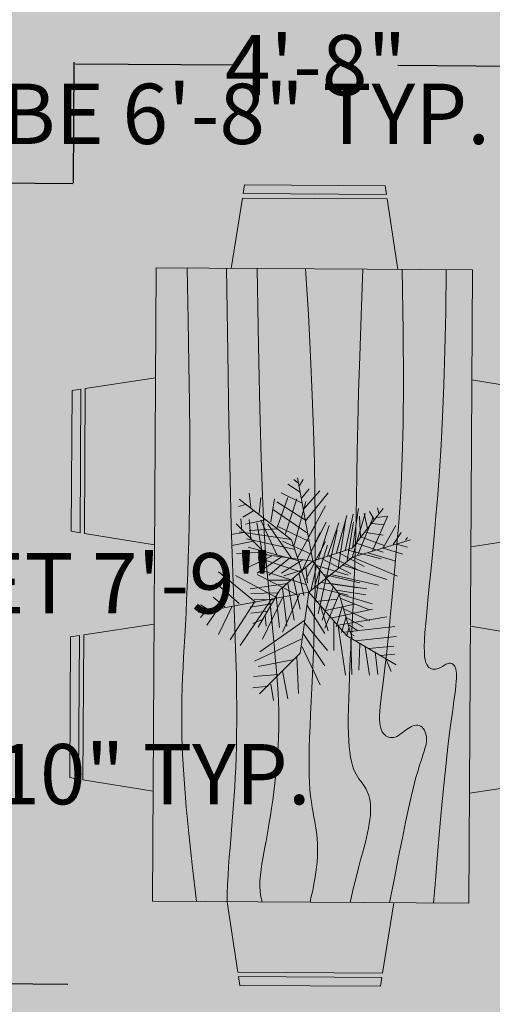
# Model space of a CAD drawing. Units: inches. Extents: x 1316 to 1777, y 813 to 1650.
# Tile 9 of 22: x 1512 to 1567, y 1319 to 1434. Entities that reach past the tile are written whole.
import ezdxf

# ---------------------------------------------------------------- set-up
doc = ezdxf.new("R2010")
doc.units = ezdxf.units.IN
doc.header["$MEASUREMENT"] = 0
for name, color, linetype, lineweight in [('A-ANNO-DIMS', 2, 'Continuous', 18), ('A-FURN-PATT', 23, 'Continuous', 13), ('furniture', 23, 'Continuous', 18), ('greenary', 106, 'Continuous', 13)]:
    doc.layers.add(name, color=color, linetype=linetype, lineweight=lineweight)
doc.layers.add('A-FLOR-PATT', color=254, linetype='Continuous', lineweight=13, true_color=0xfeeab9)
doc.styles.get("Standard").update_dxf_attribs({"font": 'arial.ttf'})
doc.dimstyles.get("Standard").update_dxf_attribs({"dimtxt": 7, "dimasz": 0.18, "dimexe": 0.18, "dimexo": 0.0625, "dimgap": 0.09, "dimtad": 0, "dimtih": 1, "dimtoh": 1, "dimzin": 0, "dimdsep": 46, "dimlunit": 3, "dimtxsty": 'Standard', "dimcen": 0.09, "dimadec": 0, "dimazin": 0, "dimtfac": 1, "dimtofl": 0, "dimtmove": 0, "dimatfit": 3, "dimfxl": 1, "dimtolj": 1, "dimtzin": 0, "dimarcsym": 0})

# ---------------------------------------------------------------- blocks, each defined once
blk = doc.blocks.new('*U13')
for p, q in [((-10.186, 53.64), (-13.084, 55.962)), ((0, 0), (-10.5, 57)), ((-9.099, 51.782), (-6.563, 55.962)), ((-8.737, 47.138), (-17.069, 52.711)), ((-7.288, 39.707), (-21.778, 46.673)), ((-7.65, 43.423), (-2.578, 49.46)), ((-5.839, 35.992), (4.667, 48.067)), ((-5.114, 27.632), (10.463, 46.673)), ((-5.114, 28.097), (-24.676, 40.636)), ((-2.941, 16.486), (8.652, 37.85)), ((27, 9), (48, 36)), ((27.127, 9.056), (31.112, 35.992)), ((44.153, 36.456), (45.239, 32.741)), ((-3.665, 19.273), (-27.574, 35.527)), ((16.259, 5.805), (23.142, 31.348)), ((22.055, 7.198), (27.489, 32.277)), ((31.836, 30.883), (32.561, 16.486)), ((35.096, 32.741), (37.27, 22.524)), ((38.719, 34.134), (41.979, 28.561)), ((43.791, 29.954), (51.036, 30.883)), ((-31.5, 4.5), (-52.5, 25.5)), ((-48.585, 21.131), (-49.309, 29.026)), ((-43.513, 28.561), (-42.427, 15.558)), ((-38.442, 26.239), (-34.819, 7.663)), ((-35.544, 28.097), (-24.314, 3.947)), ((-1.129, 6.734), (9.014, 26.704)), ((10.101, 3.483), (17.708, 26.239)), ((40.53, 25.775), (48.862, 24.846)), ((-14.533, 2.09), (-30.834, 25.31)), ((-24.314, 23.917), (-2.941, 13.7)), ((3.942, 1.625), (11.187, 24.381)), ((-47.498, 19.737), (-55.83, 18.344)), ((33.285, 16.486), (48.862, 10.913)), ((36.183, 19.737), (48.137, 17.88)), ((-40.615, 13.7), (-55.105, 10.913)), ((-20.691, 13.7), (-1.129, 4.876)), ((29.662, 12.307), (48.137, 6.269)), ((-33.37, 6.269), (-52.207, 5.34)), ((0, 0), (27, 9)), ((18.07, 5.805), (35.096, -3.483)), ((24.229, 7.663), (46.688, 1.625)), ((-28.299, 3.483), (-47.86, -5.805)), ((-21.416, 3.018), (-38.079, -8.128)), ((0, 0), (-31.5, 4.5)), ((-15.982, 2.09), (-30.11, -9.521)), ((0, 0), (-22.5, -19.5)), ((-6.563, 1.161), (-21.416, -8.128)), ((0, 0), (18, -22.5)), ((6.478, 1.625), (26.04, -8.592)), ((11.187, 3.483), (30.749, -5.805)), ((-4.752, -3.483), (-3.665, -14.629)), ((2.493, -3.019), (-1.491, -20.202)), ((1.769, -2.555), (24.229, -9.521)), ((-6.563, -5.805), (-19.967, -9.985)), ((-9.461, -8.592), (-6.201, -23.453)), ((5.029, -6.27), (2.131, -25.775)), ((7.565, -9.056), (32.198, -14.629)), ((-17.431, -15.094), (-42.789, -18.809)), ((-15.257, -12.772), (-30.11, -12.772)), ((-17.069, -15.094), (-12.721, -40.172)), ((-13.446, -11.378), (-8.737, -32.741)), ((9.014, -11.378), (3.58, -35.992)), ((12.274, -15.094), (36.907, -18.809)), ((-22.5, -19.5), (-37.5, -45)), ((-20.691, -18.345), (-17.793, -44.352)), ((14.085, -16.951), (6.478, -40.172)), ((16.259, -19.738), (36.183, -22.989)), ((-24.314, -21.596), (-42.427, -22.06)), ((-25.038, -23.918), (-22.865, -45.281)), ((18.07, -22.524), (8.289, -45.745)), ((18, -22.5), (27, -52.5)), ((18.433, -22.524), (40.53, -29.026)), ((19.157, -25.311), (38.719, -33.206)), ((-28.299, -29.026), (-42.789, -31.348)), ((-26.849, -26.24), (-40.253, -25.775)), ((20.244, -30.419), (15.897, -44.816)), ((-30.834, -34.135), (-42.427, -35.528)), ((-29.023, -30.884), (-27.936, -43.887)), ((21.331, -32.741), (39.081, -40.636)), ((-34.457, -39.708), (-40.978, -42.494)), ((-32.646, -36.921), (-31.921, -44.352)), ((22.78, -37.85), (19.519, -48.532)), ((22.78, -38.314), (34.372, -44.816)), ((24.591, -43.423), (30.749, -47.603)), ((24.591, -45.745), (23.142, -50.854)), ((26.764, -49.925), (28.213, -50.854))]:
    blk.add_line(p, q)
blk = doc.blocks.new('Dining Set - 36 x 72 in.')
for p, q in [((-22, 27.5), (-22.1562, 26.50042)), ((-22, 27.5), (-6, 27.5)), ((-5.8437, 26.49966), (-6, 27.5)), ((6, 27.5), (5.8438, 26.50042)), ((6, 27.5), (22, 27.5)), ((22.1563, 26.49966), (22, 27.5)), ((-22.2343, 26.00059), (-23.4847, 17.99762)), ((-22.2304, 26), (-5.7608, 26)), ((-5.8416, 26.5), (-22.1534, 26.5)), ((-4.5152, 17.99762), (-5.7655, 25.99926)), ((5.7657, 26.00059), (4.5153, 17.99762)), ((5.7696, 26), (22.2392, 26)), ((22.1584, 26.5), (5.8466, 26.5)), ((23.4848, 17.99762), (22.2345, 25.99926)), ((36, 18), (-36, 18)), ((-36, 18), (-36, -18)), ((36, -18), (36, 18)), ((-44.0006, 8.23428), (-35.9976, 9.48474)), ((44.0006, 8.23428), (35.9976, 9.48474)), ((-45.5, 8), (-44.5004, 8.15617)), ((-45.5, 8), (-45.5, -8)), ((-44.5, -8.15843), (-44.5, 8.15338)), ((-44, 8.23041), (-44, -8.23915)), ((44, 8.23041), (44, -8.23915)), ((44.5, -8.15843), (44.5, 8.15338)), ((45.5, 8), (44.5005, 8.15617)), ((45.5, 8), (45.5, -8)), ((-44.4997, -8.15631), (-45.5, -8)), ((-35.9976, -9.48476), (-43.9993, -8.2345)), ((35.9976, -9.48476), (43.9993, -8.2345)), ((44.4997, -8.15631), (45.5, -8)), ((-36, -18), (36, -18)), ((-22.2343, -26.0006), (-23.4847, -17.99762)), ((-4.5152, -17.99762), (-5.7655, -25.99928)), ((5.7657, -26.0006), (4.5153, -17.99762)), ((23.4848, -17.99762), (22.2345, -25.99928)), ((-22.2304, -26), (-5.7608, -26)), ((-22, -27.5), (-22.1562, -26.50044)), ((-5.8416, -26.5), (-22.1534, -26.5)), ((-5.8437, -26.49967), (-6, -27.5)), ((5.7696, -26), (22.2392, -26)), ((6, -27.5), (5.8438, -26.50044)), ((22.1584, -26.5), (5.8466, -26.5)), ((22.1563, -26.49967), (22, -27.5)), ((-22, -27.5), (-6, -27.5)), ((6, -27.5), (22, -27.5))]:
    blk.add_line(p, q)
for points in [[(-36, 15), (-31.1772, 14.97754), (-26.8079, 14.91406), (-22.8538, 14.81543), (-19.276, 14.6875), (-16.0362, 14.53613), (-13.0957, 14.36718), (-10.4159, 14.18652), (-7.9583, 14), (-5.6904, 13.81315), (-3.6035, 13.63021), (-1.6954, 13.45508), (0.0365, 13.29166), (1.5945, 13.14388), (2.9811, 13.01562), (4.1988, 12.9108), (5.25, 12.83333), (6.1393, 12.78613), (6.8802, 12.76823), (7.4883, 12.77767), (7.9792, 12.8125), (8.3685, 12.87077), (8.6719, 12.95052), (8.9049, 13.0498), (9.0833, 13.16666), (9.2205, 13.29899), (9.3216, 13.44401), (9.3895, 13.59879), (9.4271, 13.76041), (9.4373, 13.92594), (9.4232, 14.09245), (9.3875, 14.257), (9.3333, 14.41666), (9.2638, 14.56917), (9.1836, 14.71484), (9.0975, 14.85465), (9.0104, 14.98958), (8.9272, 15.1206), (8.8529, 15.2487), (8.7922, 15.37483), (8.75, 15.5), (8.7305, 15.62467), (8.7344, 15.74739), (8.7617, 15.86621), (8.8125, 15.97916), (8.8867, 16.08431), (8.9844, 16.17968), (9.1055, 16.26334), (9.25, 16.33333), (9.4189, 16.38802), (9.6172, 16.42708), (9.8506, 16.45052), (10.125, 16.45833), (10.4463, 16.45052), (10.8203, 16.42708), (11.2529, 16.38802), (11.75, 16.33333), (12.3184, 16.26318), (12.9694, 16.17838), (13.7151, 16.07991), (14.5677, 15.96875), (15.5395, 15.84586), (16.6426, 15.71224), (17.8893, 15.56884), (19.2917, 15.41666), (20.859, 15.25667), (22.5879, 15.08984), (24.4721, 14.91715), (26.5052, 14.73958), (28.6809, 14.5581), (30.9929, 14.3737), (33.4347, 14.18733), (36, 14)], [(-36, 10), (-28.9766, 10.14274), (-23.1725, 10.20442), (-18.4241, 10.19775), (-14.5677, 10.13541), (-11.4399, 10.03011), (-8.877, 9.89453), (-6.7154, 9.74137), (-4.7917, 9.58333), (-2.9698, 9.43082), (-1.2246, 9.28515), (0.4415, 9.14534), (2.026, 9.01041), (3.5266, 8.87939), (4.9408, 8.7513), (6.266, 8.62516), (7.5, 8.5), (8.6411, 8.37549), (9.6914, 8.2539), (10.6538, 8.13818), (11.5312, 8.03125), (12.3267, 7.93603), (13.043, 7.85547), (13.6831, 7.79248), (14.25, 7.75), (14.7471, 7.7303), (15.1797, 7.73307), (15.5537, 7.75732), (15.875, 7.80208), (16.1494, 7.86637), (16.3828, 7.94922), (16.5811, 8.04964), (16.75, 8.16666), (16.8944, 8.29915), (17.0143, 8.44531), (17.1089, 8.60319), (17.1771, 8.77083), (17.218, 8.94629), (17.2305, 9.1276), (17.2137, 9.31282), (17.1667, 9.5), (17.0895, 9.6875), (16.987, 9.875), (16.8649, 10.0625), (16.7292, 10.25), (16.5856, 10.4375), (16.4401, 10.625), (16.2985, 10.8125), (16.1667, 11), (16.05, 11.18733), (15.9518, 11.3737), (15.8752, 11.5581), (15.8229, 11.73958), (15.798, 11.91715), (15.8034, 12.08984), (15.842, 12.25667), (15.9167, 12.41666), (16.0295, 12.56836), (16.1784, 12.70833), (16.3605, 12.83268), (16.5729, 12.9375), (16.8127, 13.01888), (17.0768, 13.07291), (17.3625, 13.0957), (17.6667, 13.08333), (17.9894, 13.03312), (18.3418, 12.94726), (18.7382, 12.82918), (19.1927, 12.68229), (19.7195, 12.51001), (20.3327, 12.31575), (21.0465, 12.10294), (21.875, 11.875), (22.8357, 11.63354), (23.959, 11.37304), (25.2786, 11.08618), (26.8282, 10.76562), (28.6414, 10.40405), (30.752, 9.99414), (33.1936, 9.52856), (36, 9)], [(-36, 5.5), (-30.7157, 5.3348), (-26.069, 5.20963), (-21.9946, 5.11767), (-18.4271, 5.05208), (-15.3009, 5.00602), (-12.5508, 4.97265), (-10.1112, 4.94515), (-7.9167, 4.91666), (-5.909, 4.88167), (-4.0586, 4.83984), (-2.3429, 4.79215), (-0.7396, 4.73958), (0.7739, 4.6831), (2.22, 4.6237), (3.6213, 4.56233), (5, 4.5), (6.373, 4.43782), (7.7344, 4.3776), (9.0723, 4.32129), (10.375, 4.27083), (11.6309, 4.22819), (12.8281, 4.19531), (13.9551, 4.17415), (15, 4.16666), (15.954, 4.17448), (16.819, 4.19791), (17.6001, 4.23698), (18.3021, 4.29166), (18.9299, 4.36198), (19.4883, 4.44791), (19.9823, 4.54948), (20.4167, 4.66666), (20.7969, 4.79899), (21.1302, 4.94401), (21.4245, 5.09879), (21.6875, 5.26041), (21.9271, 5.42594), (22.1511, 5.59245), (22.3672, 5.757), (22.5834, 5.91666), (22.8065, 6.06868), (23.0404, 6.21093), (23.2879, 6.34147), (23.5521, 6.45833), (23.8358, 6.55957), (24.142, 6.64323), (24.4735, 6.70735), (24.8334, 6.75), (25.2235, 6.76969), (25.642, 6.76692), (26.0858, 6.74267), (26.5521, 6.69791), (27.0379, 6.63362), (27.5404, 6.55078), (28.0565, 6.45036), (28.5834, 6.33333), (29.1242, 6.19987), (29.7071, 6.04687), (30.3661, 5.87044), (31.1354, 5.66666), (32.0493, 5.43164), (33.142, 5.16146), (34.4475, 4.85221), (36, 4.5)], [(-36, -1), (-30.7915, -0.6591), (-26.0195, -0.38216), (-21.6519, -0.16284), (-17.6563, 0.00521), (-14.0005, 0.12833), (-10.6523, 0.21289), (-7.5796, 0.26522), (-4.75, 0.29166), (-2.134, 0.29793), (0.2878, 0.28711), (2.5317, 0.26163), (4.6146, 0.22396), (6.5529, 0.17651), (8.3633, 0.12174), (10.0623, 0.06209), (11.6667, 0), (13.1899, -0.06201), (14.6341, -0.1211), (15.9982, -0.17432), (17.2813, -0.21875), (18.4823, -0.25147), (19.6003, -0.26953), (20.6343, -0.27002), (21.5834, -0.25), (22.4481, -0.20768), (23.2357, -0.14584), (23.9549, -0.06836), (24.6146, 0.02083), (25.2235, 0.11784), (25.7904, 0.21875), (26.3241, 0.31966), (26.8334, 0.41666), (27.3265, 0.50618), (27.8099, 0.58593), (28.2894, 0.65397), (28.7709, 0.70833), (29.2601, 0.74707), (29.763, 0.76823), (30.2855, 0.76985), (30.8334, 0.75), (31.4088, 0.70784), (31.9994, 0.64713), (32.589, 0.57275), (33.1615, 0.48958), (33.7008, 0.4025), (34.1908, 0.3164), (34.6153, 0.23616), (34.9584, 0.16666), (35.2099, 0.11165), (35.3848, 0.07031), (35.504, 0.04069), (35.5886, 0.02083), (35.6594, 0.00879), (35.7377, 0.0026), (35.8442, 0.00032), (36, 0)], [(-36, -6.5), (-27.1843, -6.31267), (-20.084, -6.1263), (-14.469, -5.9419), (-10.1094, -5.76042), (-6.7752, -5.58285), (-4.2363, -5.41016), (-2.2629, -5.24333), (-0.625, -5.08334), (0.8708, -4.93099), (2.2715, -4.78646), (3.5872, -4.64974), (4.8281, -4.52084), (6.0046, -4.39974), (7.127, -4.28646), (8.2053, -4.18099), (9.25, -4.08334), (10.2705, -3.99382), (11.2734, -3.91407), (12.2647, -3.84603), (13.25, -3.79167), (14.2354, -3.75293), (15.2266, -3.73177), (16.2295, -3.73015), (17.25, -3.75), (18.2912, -3.79248), (19.3451, -3.85547), (20.4009, -3.93604), (21.4479, -4.03125), (22.4754, -4.13819), (23.4727, -4.25391), (24.4289, -4.37549), (25.3334, -4.5), (26.1785, -4.62492), (26.9694, -4.74935), (27.7145, -4.87281), (28.4219, -4.99479), (29.1, -5.11483), (29.7572, -5.23242), (30.4016, -5.34709), (31.0417, -5.45834), (31.6837, -5.56437), (32.3262, -5.65821), (32.9658, -5.73153), (33.599, -5.77604), (34.2224, -5.78345), (34.8327, -5.74545), (35.4264, -5.65373), (36, -5.5)], [(-36, -10), (-26.4022, -9.81299), (-18.4675, -9.62891), (-11.9839, -9.45069), (-6.7396, -9.28125), (-2.5226, -9.12354), (0.8789, -8.98047), (3.6769, -8.85498), (6.0833, -8.75), (8.2767, -8.66765), (10.3021, -8.60677), (12.1712, -8.56543), (13.8958, -8.54167), (15.4876, -8.53353), (16.9583, -8.53907), (18.3197, -8.55632), (19.5834, -8.58334), (20.7616, -8.61841), (21.8685, -8.66081), (22.9188, -8.71004), (23.9271, -8.76563), (24.9081, -8.82707), (25.8763, -8.89388), (26.8465, -8.96558), (27.8334, -9.04167), (28.8474, -9.12118), (29.8828, -9.20117), (30.93, -9.27824), (31.9792, -9.34896), (33.0205, -9.40991), (34.0443, -9.45768), (35.0407, -9.48885), (36, -9.5)], [(-36, -14.5), (-30.0881, -14.33513), (-25.0332, -14.21224), (-20.7312, -14.12647), (-17.0781, -14.07292), (-13.97, -14.04671), (-11.3027, -14.04297), (-8.9724, -14.05681), (-6.875, -14.08334), (-4.9224, -14.11833), (-3.0905, -14.16016), (-1.3709, -14.20785), (0.2448, -14.26042), (1.7647, -14.3169), (3.1973, -14.3763), (4.5507, -14.43767), (5.8333, -14.5), (7.0554, -14.5621), (8.235, -14.62175), (9.3922, -14.67652), (10.5469, -14.72396), (11.7192, -14.76164), (12.929, -14.78711), (14.1965, -14.79794), (15.5417, -14.79167), (16.9933, -14.76424), (18.6152, -14.70508), (20.4804, -14.60197), (22.6615, -14.44271), (25.2312, -14.21509), (28.2624, -13.9069), (31.8277, -13.50594), (36, -13)]]:
    blk.add_lwpolyline(points)
blk = doc.blocks.new('dining area')
at = {"layer": 'furniture', "xscale": 0.6659924291999282, "yscale": 0.6659924291999282, "zscale": 0.6659924291999282, "rotation": 90}
blk.add_blockref('Dining Set - 36 x 72 in.', (-0.439, 20.507), dxfattribs=at)
blk = doc.blocks.new('*D30')
at = {"layer": 'A-ANNO-DIMS', "color": 0, "lineweight": -2, "transparency": 16777216}
for p, q in [((1386.15, 1434.7), (1386.15, 1422.58)), ((1466.18, 1434.7), (1466.18, 1422.58)), ((1386.33, 1422.76), (1466, 1422.76)), ((1466.18, 1422.76), (1466.36, 1422.76))]:
    blk.add_line(p, q, dxfattribs=at)
at = {"layer": 'A-ANNO-DIMS', "color": 0, "transparency": 16777216}
for points in [[(1386.33, 1422.79), (1386.33, 1422.73), (1386.15, 1422.76)], [(1466, 1422.79), (1466, 1422.73), (1466.18, 1422.76)]]:
    blk.add_solid(points, dxfattribs=at)
at = {"layer": 'Defpoints', "color": 0, "transparency": 16777216}
for p in [(1386.15, 1434.76), (1466.18, 1434.76), (1466.18, 1422.76)]:
    blk.add_point(p, dxfattribs=at)
at = {"layer": 'A-ANNO-DIMS', "color": 0, "transparency": 16777216, "insert": (1518.08, 1422.76), "char_height": 7, "attachment_point": 5}
blk.add_mtext('\\A1;WARDROBE 6\'-8" TYP.', dxfattribs=at)
blk = doc.blocks.new('*D36')
at = {"layer": 'A-ANNO-DIMS', "color": 0, "lineweight": -2, "transparency": 16777216}
for p, q in [((1416.11, 1349.39), (1416.11, 1345.95)), ((1438.26, 1349.39), (1438.26, 1345.95)), ((1416.29, 1346.13), (1438.08, 1346.13)), ((1438.26, 1346.13), (1438.44, 1346.13))]:
    blk.add_line(p, q, dxfattribs=at)
at = {"layer": 'A-ANNO-DIMS', "color": 0, "transparency": 16777216}
for points in [[(1416.29, 1346.16), (1416.29, 1346.1), (1416.11, 1346.13)], [(1438.08, 1346.16), (1438.08, 1346.1), (1438.26, 1346.13)]]:
    blk.add_solid(points, dxfattribs=at)
at = {"layer": 'Defpoints', "color": 0, "transparency": 16777216}
for p in [(1416.11, 1349.46), (1438.26, 1349.46), (1438.26, 1346.13)]:
    blk.add_point(p, dxfattribs=at)
at = {"layer": 'A-ANNO-DIMS', "color": 0, "transparency": 16777216, "insert": (1493.43, 1346.13), "char_height": 7, "attachment_point": 5}
blk.add_mtext('\\A1;WALL BASIN 1\'-10" TYP.', dxfattribs=at)
blk = doc.blocks.new('*D40')
at = {"layer": 'A-ANNO-DIMS', "color": 0, "lineweight": -2, "transparency": 16777216}
for p, q in [((1388.84, 1302.16), (1388.84, 1312.14)), ((1389.02, 1311.96), (1454.4, 1311.96)), ((1454.58, 1302.16), (1454.58, 1312.14)), ((1454.58, 1311.96), (1454.76, 1311.96))]:
    blk.add_line(p, q, dxfattribs=at)
at = {"layer": 'A-ANNO-DIMS', "color": 0, "transparency": 16777216}
for points in [[(1389.02, 1311.99), (1389.02, 1311.93), (1388.84, 1311.96)], [(1454.4, 1311.99), (1454.4, 1311.93), (1454.58, 1311.96)]]:
    blk.add_solid(points, dxfattribs=at)
at = {"layer": 'Defpoints', "color": 0, "transparency": 16777216}
for p in [(1454.58, 1311.96), (1388.84, 1302.1), (1454.58, 1302.1)]:
    blk.add_point(p, dxfattribs=at)
at = {"layer": 'A-ANNO-DIMS', "color": 0, "transparency": 16777216, "insert": (1507.74, 1311.96), "char_height": 7, "attachment_point": 5}
blk.add_mtext('\\A1;KITCHEN SINK 5\'-5 1/2"', dxfattribs=at)
blk = doc.blocks.new('*D48')
at = {"layer": 'A-ANNO-DIMS', "color": 0, "lineweight": -2, "transparency": 16777216}
for p, q in [((1504.09, 1414.55), (1503.83, 1371.99)), ((1517.96, 1414.64), (1503.91, 1414.73)), ((1503.52, 1322.01), (1503.78, 1364.57)), ((1517.39, 1321.74), (1503.34, 1321.83))]:
    blk.add_line(p, q, dxfattribs=at)
at = {"layer": 'A-ANNO-DIMS', "color": 0, "transparency": 16777216}
for points in [[(1504.06, 1414.55), (1504.12, 1414.55), (1504.09, 1414.73)], [(1503.49, 1322.01), (1503.55, 1322.01), (1503.52, 1321.83)]]:
    blk.add_solid(points, dxfattribs=at)
at = {"layer": 'Defpoints', "color": 0, "transparency": 16777216}
for p in [(1518.02, 1414.64), (1503.52, 1321.83), (1517.46, 1321.74)]:
    blk.add_point(p, dxfattribs=at)
at = {"layer": 'A-ANNO-DIMS', "color": 0, "transparency": 16777216, "insert": (1503.81, 1368.28), "char_height": 7, "attachment_point": 5}
blk.add_mtext('\\A1;DINING SET 7\'-9"', dxfattribs=at)
blk = doc.blocks.new('*D49')
at = {"layer": 'A-ANNO-DIMS', "color": 0, "lineweight": -2, "transparency": 16777216}
for p, q in [((1518.03, 1414.71), (1518.11, 1428.76)), ((1518.29, 1428.58), (1536.65, 1428.46)), ((1574.08, 1428.24), (1555.72, 1428.35)), ((1574.17, 1414.36), (1574.26, 1428.41))]:
    blk.add_line(p, q, dxfattribs=at)
at = {"layer": 'A-ANNO-DIMS', "color": 0, "transparency": 16777216}
for points in [[(1518.29, 1428.61), (1518.29, 1428.55), (1518.11, 1428.58)], [(1574.08, 1428.27), (1574.08, 1428.21), (1574.26, 1428.23)]]:
    blk.add_solid(points, dxfattribs=at)
at = {"layer": 'Defpoints', "color": 0, "transparency": 16777216}
for p in [(1518.11, 1428.58), (1518.02, 1414.64), (1574.17, 1414.3)]:
    blk.add_point(p, dxfattribs=at)
at = {"layer": 'A-ANNO-DIMS', "color": 0, "transparency": 16777216, "insert": (1546.18, 1428.41), "char_height": 7, "attachment_point": 5}
blk.add_mtext('\\A1;4\'-8"', dxfattribs=at)

msp = doc.modelspace()

# ---------------------------------------------------------------- hatches: boundary and pattern name
at = {"layer": 'A-FLOR-PATT'}
h = msp.add_hatch(color=256, dxfattribs=at)
h.dxf.hatch_style = 1
h.paths.add_polyline_path([(1567.673, 1281.369), (1651.673, 1281.369), (1651.673, 1365.369), (1597.673, 1365.369), (1597.673, 1429.869), (1570.345, 1429.869), (1570.345, 1471.869), (1510.345, 1471.869), (1510.345, 1429.869), (1444.564, 1429.869), (1444.564, 1322.882), (1444.564, 1300.088), (1510.564, 1300.088), (1510.564, 1295.094), (1510.564, 1240.869), (1386.064, 1240.869), (1386.064, 1171.185), (1400.961, 1171.185), (1400.961, 1106.742), (1386.064, 1106.742), (1386.064, 1072.869), (1510.564, 1072.869), (1510.564, 1040.173), (1541.068, 1040.173, -0.367085), (1572.764, 1069.547), (1572.764, 1069.579), (1574.225, 1069.579), (1574.225, 1040.173), (1616.037, 1040.173), (1616.037, 1086.627), (1616.037, 1103.705), (1613.066, 1105.235), (1616.037, 1106.686), (1616.037, 1123.869), (1567.673, 1123.869)])
h.paths.add_polyline_path([(1508.987, 1198.018), (1511.117, 1198.018), (1511.117, 1200.148), (1532.595, 1200.148), (1532.595, 1198.018), (1534.725, 1198.018), (1534.725, 1176.008), (1530.465, 1176.008), (1530.465, 1176.718), (1513.247, 1176.718), (1513.247, 1176.008), (1508.987, 1176.008)], flags=16)
h.paths.add_polyline_path([(1505.979, 1151.315), (1521.504, 1151.315), (1521.504, 1123.623), (1505.979, 1123.623)], flags=16)
h.paths.add_polyline_path([(1507.734, 1150.101, -1), (1506.932, 1150.101, -1)], flags=0)
h.paths.add_polyline_path([(1512.288, 1138.353), (1512.28, 1138.392), (1512.219, 1138.376)], flags=0)
h.paths.add_polyline_path([(1511.539, 1138.926), (1511.802, 1138.967), (1511.817, 1139.27), (1511.607, 1139.246)], flags=0)
h.paths.add_polyline_path([(1513.745, 1140.234), (1513.68, 1139.885), (1514.014, 1140.045), (1513.855, 1140.308)], flags=0)
h.paths.add_polyline_path([(1513.759, 1139.089), (1514.005, 1139.255), (1513.807, 1139.483), (1513.564, 1139.327)], flags=0)
h.paths.add_polyline_path([(1514.219, 1138.385), (1514.336, 1138.33), (1514.544, 1138.32), (1514.802, 1138.874), (1514.451, 1138.716)], flags=0)
h.paths.add_polyline_path([(1514.577, 1137.439), (1514.573, 1137.4), (1514.699, 1137.4), (1514.696, 1137.402)], flags=0)
h.paths.add_polyline_path([(1512.26, 1136.199), (1512.199, 1136.399), (1512.032, 1136.325), (1512.095, 1136.101), (1512.257, 1136.192)], flags=0)
h.paths.add_polyline_path([(1512.644, 1137.274), (1512.356, 1137.23), (1512.432, 1137.049), (1512.703, 1137.093)], flags=0)
h.paths.add_polyline_path([(1513.049, 1137.593), (1512.979, 1137.8), (1512.843, 1137.757), (1512.887, 1137.556)], flags=0)
h.paths.add_polyline_path([(1513.269, 1138.556), (1513.571, 1137.962), (1513.459, 1136.814), (1513.212, 1137.878), (1513.032, 1138.443)], flags=0)
h.paths.add_polyline_path([(1514.891, 1136.377), (1514.696, 1136.401), (1514.683, 1136.246), (1514.87, 1136.165)], flags=0)
h.paths.add_polyline_path([(1514.142, 1137.293), (1514.047, 1136.743), (1514.27, 1136.751), (1514.328, 1137.265)], flags=0)
h.paths.add_polyline_path([(1515.362, 1138.976), (1515.334, 1138.638), (1515.596, 1138.588), (1515.627, 1138.932)], flags=0)
h.paths.add_polyline_path([(1537.285, 1177.912), (1537.995, 1177.912), (1537.995, 1195.13), (1537.285, 1195.13), (1537.285, 1199.39), (1559.295, 1199.39), (1559.295, 1197.26), (1561.425, 1197.26), (1561.425, 1175.782), (1559.295, 1175.782), (1559.295, 1173.652), (1559.379, 1173.652), (1559.379, 1171.514), (1561.517, 1171.514), (1561.517, 1098.819), (1559.379, 1098.819), (1559.379, 1096.68), (1537.285, 1096.68), (1537.285, 1100.957), (1537.997, 1100.957), (1537.997, 1169.376), (1537.285, 1169.376), (1537.285, 1173.652)], flags=16)
h.paths.add_polyline_path([(1518.623, 1345.565), (1519.133, 1345.48), (1519.133, 1345.485), (1518.623, 1345.567)], flags=16)
h.paths.add_polyline_path([(1518.798, 1374.15), (1519.308, 1374.064), (1519.308, 1374.069), (1518.798, 1374.152)], flags=16)
h.paths.add_polyline_path([(1537.764, 1413.501), (1537.678, 1412.991), (1537.683, 1412.991), (1537.766, 1413.501)], flags=16)
h.paths.add_polyline_path([(1572.905, 1373.821), (1573.927, 1373.975), (1574.027, 1390.309), (1573.007, 1390.475), (1573.007, 1390.475)], flags=16)
h.paths.add_polyline_path([(1572.73, 1345.237), (1573.752, 1345.39), (1573.852, 1361.724), (1572.832, 1361.89), (1572.832, 1361.89)], flags=16)
h.paths.add_polyline_path([(1537.211, 1322.643), (1537.364, 1321.621), (1553.698, 1321.521), (1553.864, 1322.541)], flags=16)
h.paths.add_polyline_path([(1535.908, 1331.328), (1527.214, 1331.382), (1527.664, 1404.885), (1564.416, 1404.66), (1563.966, 1331.157), (1555.273, 1331.21), (1553.947, 1323.051), (1537.134, 1323.154)], flags=16)
h.paths.add_polyline_path([(1536.15, 1336.503), (1536.235, 1337.572), (1536.323, 1338.628), (1536.411, 1339.663), (1536.495, 1340.67), (1536.574, 1341.66), (1536.648, 1342.648), (1536.717, 1343.649), (1536.78, 1344.678), (1536.837, 1345.75), (1536.913, 1347.475), (1536.93, 1348.082), (1536.867, 1346.314), (1536.754, 1344.188), (1536.619, 1342.219), (1536.495, 1340.67), (1536.411, 1339.663), (1536.323, 1338.628), (1536.235, 1337.572), (1536.15, 1336.503), (1536.071, 1335.432), (1536.002, 1334.37), (1535.917, 1332.754), (1535.909, 1332.308), (1535.964, 1333.78), (1536.071, 1335.432)], flags=0)
h.paths.add_polyline_path([(1540.412, 1338.345), (1540.539, 1339.037), (1540.667, 1339.758), (1540.798, 1340.518), (1540.93, 1341.325), (1541.063, 1342.187), (1541.196, 1343.109), (1541.326, 1344.085), (1541.45, 1345.102), (1541.566, 1346.15), (1541.669, 1347.219), (1541.758, 1348.296), (1541.829, 1349.371), (1541.879, 1350.434), (1541.906, 1351.476), (1541.91, 1352.5), (1541.895, 1353.512), (1541.861, 1354.518), (1541.812, 1355.524), (1541.749, 1356.537), (1541.674, 1357.561), (1541.551, 1359.062), (1541.495, 1359.67), (1541.589, 1358.603), (1541.721, 1356.977), (1541.846, 1354.98), (1541.912, 1352.982), (1541.903, 1350.951), (1541.806, 1348.87), (1541.628, 1346.713), (1541.396, 1344.612), (1541.135, 1342.656), (1540.872, 1340.947), (1540.617, 1339.466), (1540.412, 1338.345), (1540.288, 1337.675), (1540.166, 1337.018), (1540.049, 1336.365), (1539.937, 1335.71), (1539.837, 1335.055), (1539.758, 1334.403), (1539.709, 1333.756), (1539.697, 1333.12), (1539.751, 1332.162), (1539.822, 1331.89), (1539.691, 1332.775), (1539.714, 1334.035), (1539.867, 1335.303), (1540.085, 1336.577), (1540.288, 1337.675)], flags=0)
h.paths.add_polyline_path([(1545.599, 1331.584), (1545.601, 1331.617), (1545.614, 1331.689), (1545.737, 1332.197), (1545.767, 1332.332), (1545.84, 1332.681), (1545.925, 1333.114), (1546.016, 1333.614), (1546.108, 1334.164), (1546.196, 1334.748), (1546.276, 1335.349), (1546.342, 1335.952), (1546.388, 1336.539), (1546.412, 1337.098), (1546.414, 1337.632), (1546.395, 1338.145), (1546.359, 1338.645), (1546.306, 1339.137), (1546.24, 1339.627), (1546.161, 1340.121), (1546.073, 1340.625), (1545.888, 1341.63), (1545.718, 1342.621), (1545.547, 1343.945), (1545.432, 1345.534), (1545.404, 1347.402), (1545.418, 1348.013), (1545.411, 1346.957), (1545.425, 1345.988), (1545.463, 1345.105), (1545.521, 1344.301), (1545.596, 1343.566), (1545.683, 1342.892), (1545.778, 1342.27), (1545.877, 1341.691), (1545.977, 1341.145), (1546.133, 1340.297), (1546.327, 1339.075), (1546.434, 1337.615), (1546.377, 1336.279), (1546.246, 1335.079), (1546.032, 1333.665), (1545.84, 1332.681), (1545.767, 1332.332)], flags=0)
h.paths.add_polyline_path([(1551.803, 1337.656), (1551.963, 1338.25), (1552.102, 1338.801), (1552.225, 1339.338), (1552.331, 1339.865), (1552.418, 1340.377), (1552.487, 1340.873), (1552.536, 1341.348), (1552.563, 1341.801), (1552.569, 1342.228), (1552.551, 1342.627), (1552.51, 1342.995), (1552.446, 1343.333), (1552.363, 1343.646), (1552.261, 1343.937), (1552.144, 1344.207), (1552.012, 1344.461), (1551.868, 1344.7), (1551.746, 1344.882), (1550.887, 1346.052), (1550.428, 1347.126), (1550.183, 1348.353), (1550.048, 1349.632), (1549.978, 1351.224), (1549.974, 1353.141), (1549.989, 1353.748), (1549.975, 1352.682), (1549.977, 1351.708), (1549.996, 1350.825), (1550.031, 1350.027), (1550.082, 1349.31), (1550.15, 1348.669), (1550.234, 1348.098), (1550.335, 1347.593), (1550.452, 1347.149), (1550.584, 1346.76), (1550.73, 1346.419), (1550.887, 1346.117), (1551.05, 1345.848), (1551.217, 1345.602), (1551.386, 1345.372), (1551.553, 1345.151), (1552, 1344.537), (1552.454, 1343.495), (1552.591, 1342.266), (1552.509, 1340.905), (1552.246, 1339.367), (1551.925, 1338.101), (1551.619, 1336.984), (1551.406, 1336.2), (1551.01, 1334.699), (1550.877, 1334.155), (1551.264, 1335.677), (1551.619, 1336.984)], flags=0)
h.paths.add_polyline_path([(1558.642, 1348.348), (1558.795, 1348.811), (1558.918, 1349.215), (1559.008, 1349.575), (1559.061, 1349.904), (1559.076, 1350.214), (1559.054, 1350.506), (1559.001, 1350.776), (1558.919, 1351.021), (1558.814, 1351.239), (1558.688, 1351.425), (1558.546, 1351.578), (1558.392, 1351.694), (1558.229, 1351.772), (1558.059, 1351.812), (1557.882, 1351.819), (1557.701, 1351.794), (1557.515, 1351.742), (1557.327, 1351.665), (1557.136, 1351.566), (1556.944, 1351.448), (1556.752, 1351.315), (1556.742, 1351.307), (1556.175, 1350.878), (1555.982, 1350.741), (1555.79, 1350.618), (1555.103, 1350.248), (1554.019, 1350.696), (1553.658, 1351.734), (1553.592, 1352.861), (1553.705, 1354.248), (1553.753, 1354.657), (1553.685, 1354.004), (1553.638, 1353.425), (1553.615, 1352.918), (1553.615, 1352.476), (1553.637, 1352.094), (1553.681, 1351.766), (1553.745, 1351.485), (1553.828, 1351.246), (1553.929, 1351.043), (1554.048, 1350.87), (1554.182, 1350.722), (1554.33, 1350.599), (1554.491, 1350.501), (1554.662, 1350.43), (1554.841, 1350.388), (1555.026, 1350.374), (1555.215, 1350.39), (1555.406, 1350.437), (1555.598, 1350.514), (1555.79, 1350.618), (1555.982, 1350.741), (1556.175, 1350.878), (1556.367, 1351.024), (1556.559, 1351.171), (1556.752, 1351.315), (1556.944, 1351.448), (1557.136, 1351.566), (1557.327, 1351.665), (1558.043, 1351.957), (1558.894, 1351.316), (1559.137, 1350.09), (1558.886, 1349.087), (1558.642, 1348.348), (1558.463, 1347.812), (1558.261, 1347.187), (1558.039, 1346.459), (1557.677, 1345.175), (1557.549, 1344.636), (1557.909, 1346.03), (1558.329, 1347.408)], flags=0)
h.paths.add_polyline_path([(1562.145, 1353.919), (1562.25, 1354.68), (1562.341, 1355.344), (1562.416, 1355.924), (1562.475, 1356.431), (1562.518, 1356.872), (1562.544, 1357.254), (1562.554, 1357.582), (1562.548, 1357.862), (1562.525, 1358.1), (1562.486, 1358.303), (1562.432, 1358.476), (1562.361, 1358.624), (1562.277, 1358.748), (1562.18, 1358.848), (1562.073, 1358.925), (1561.958, 1358.977), (1561.837, 1359.006), (1561.711, 1359.011), (1561.584, 1358.992), (1561.456, 1358.949), (1561.342, 1358.895), (1560.78, 1358.554), (1560.631, 1358.473), (1560.474, 1358.403), (1560.311, 1358.348), (1559.637, 1358.207), (1558.973, 1358.904), (1558.816, 1360.002), (1558.804, 1361.236), (1558.83, 1361.674), (1558.807, 1360.917), (1558.813, 1360.297), (1558.845, 1359.795), (1558.902, 1359.397), (1558.982, 1359.087), (1559.082, 1358.849), (1559.2, 1358.666), (1559.334, 1358.525), (1559.482, 1358.421), (1559.639, 1358.351), (1559.804, 1358.311), (1559.973, 1358.3), (1560.143, 1358.313), (1560.311, 1358.348), (1560.474, 1358.403), (1560.631, 1358.473), (1560.78, 1358.554), (1560.923, 1358.641), (1561.061, 1358.729), (1561.196, 1358.813), (1561.382, 1358.92), (1561.342, 1358.895), (1561.972, 1359.194), (1562.536, 1358.367), (1562.56, 1357.311), (1562.455, 1356.226), (1562.323, 1355.206), (1562.145, 1353.919), (1562.026, 1353.049), (1561.815, 1351.457), (1561.752, 1350.933), (1561.948, 1352.479)], flags=0)
h.paths.add_polyline_path([(1572.764, 1069.547, 0.367085), (1541.068, 1040.173), (1572.764, 1040.173)], flags=17)
h.paths.add_polyline_path([(1572.764, 1040.173), (1541.068, 1040.173, 0.0299535), (1540.829, 1036.182), (1540.829, 1031.173), (1574.225, 1031.173), (1574.225, 1036.182), (1572.764, 1036.182)])
at = {"layer": 'A-FURN-PATT'}
h = msp.add_hatch(color=256, dxfattribs=at)
h.dxf.hatch_style = 1
h.paths.add_polyline_path([(1527.586, 1392.108), (1519.411, 1390.882), (1519.308, 1374.069), (1527.467, 1372.743)])
h.paths.add_polyline_path([(1527.411, 1363.523), (1519.236, 1362.297), (1519.133, 1345.485), (1527.293, 1344.158)])
h.paths.add_polyline_path([(1572.322, 1361.973), (1564.163, 1363.299), (1564.044, 1343.934), (1572.219, 1345.16)])
h.paths.add_polyline_path([(1572.497, 1390.557), (1564.337, 1391.883), (1564.219, 1372.519), (1572.394, 1373.745)])
h.paths.add_polyline_path([(1555.273, 1331.21), (1535.908, 1331.328), (1537.134, 1323.154), (1553.947, 1323.051)])
h.paths.add_polyline_path([(1554.496, 1412.889), (1537.683, 1412.991), (1536.357, 1404.832), (1555.722, 1404.714)])
h.paths.add_polyline_path([(1554.266, 1414.421), (1537.932, 1414.521), (1537.766, 1413.501), (1554.419, 1413.399)])
h.paths.add_polyline_path([(1518.9, 1390.805), (1517.878, 1390.652), (1517.778, 1374.318), (1518.798, 1374.152)])
h.paths.add_polyline_path([(1518.725, 1362.221), (1517.703, 1362.067), (1517.603, 1345.733), (1518.623, 1345.567)])
h.paths.add_polyline_path([(1553.864, 1322.541), (1537.211, 1322.643), (1537.364, 1321.621), (1553.698, 1321.521)])
h.paths.add_polyline_path([(1573.852, 1361.724), (1572.832, 1361.89), (1572.73, 1345.237), (1573.752, 1345.39)])
h.paths.add_polyline_path([(1574.027, 1390.309), (1573.007, 1390.475), (1572.905, 1373.821), (1573.927, 1373.975)])
h = msp.add_hatch(color=256, dxfattribs=at)
h.dxf.hatch_style = 1
h.paths.add_polyline_path([(1531.237, 1404.863), (1531.368, 1398.827), (1531.462, 1393.666), (1531.523, 1389.273), (1531.555, 1385.544), (1531.562, 1382.37), (1531.549, 1379.647), (1531.521, 1377.269), (1531.48, 1375.127), (1531.433, 1373.134), (1531.378, 1371.264), (1531.319, 1369.509), (1531.255, 1367.86), (1531.188, 1366.309), (1531.119, 1364.847), (1531.047, 1363.465), (1530.976, 1362.156), (1530.905, 1360.909), (1530.836, 1359.705), (1530.773, 1358.524), (1530.718, 1357.346), (1530.672, 1356.149), (1530.638, 1354.914), (1530.619, 1353.62), (1530.617, 1352.247), (1530.636, 1350.765), (1530.687, 1349.109), (1530.78, 1347.204), (1530.929, 1344.976), (1531.146, 1342.352), (1531.441, 1339.255), (1531.828, 1335.613), (1532.319, 1331.35), (1539.975, 1331.304), (1539.822, 1331.89), (1539.732, 1332.497), (1539.697, 1333.12), (1539.709, 1333.756), (1539.758, 1334.403), (1539.837, 1335.055), (1539.937, 1335.71), (1540.049, 1336.365), (1540.166, 1337.018), (1540.288, 1337.675), (1540.412, 1338.345), (1540.539, 1339.037), (1540.667, 1339.758), (1540.798, 1340.518), (1540.93, 1341.325), (1541.063, 1342.187), (1541.196, 1343.109), (1541.326, 1344.085), (1541.45, 1345.102), (1541.566, 1346.15), (1541.669, 1347.219), (1541.758, 1348.296), (1541.829, 1349.371), (1541.879, 1350.434), (1541.906, 1351.476), (1541.91, 1352.5), (1541.895, 1353.512), (1541.861, 1354.518), (1541.812, 1355.524), (1541.749, 1356.537), (1541.674, 1357.561), (1541.589, 1358.603), (1541.495, 1359.67), (1541.395, 1360.772), (1541.286, 1361.918), (1541.17, 1363.12), (1541.046, 1364.388), (1540.914, 1365.732), (1540.776, 1367.163), (1540.623, 1368.754), (1539.104, 1368.474), (1539.15, 1368.546), (1539.213, 1368.494), (1540.624, 1368.754), (1540.476, 1370.364), (1540.318, 1372.38), (1540.158, 1374.973), (1539.997, 1378.377), (1539.839, 1382.829), (1539.686, 1388.563), (1539.54, 1395.812), (1539.404, 1404.813)])
h.paths.add_polyline_path([(1527.664, 1404.885), (1527.214, 1331.382), (1532.319, 1331.35), (1531.828, 1335.613), (1531.441, 1339.255), (1531.146, 1342.352), (1530.929, 1344.976), (1530.78, 1347.204), (1530.687, 1349.109), (1530.636, 1350.765), (1530.617, 1352.247), (1530.619, 1353.62), (1530.638, 1354.914), (1530.672, 1356.149), (1530.718, 1357.346), (1530.773, 1358.524), (1530.836, 1359.705), (1530.905, 1360.909), (1530.976, 1362.156), (1531.047, 1363.465), (1531.119, 1364.847), (1531.188, 1366.309), (1531.255, 1367.86), (1531.319, 1369.509), (1531.378, 1371.264), (1531.433, 1373.134), (1531.48, 1375.127), (1531.521, 1377.269), (1531.549, 1379.647), (1531.562, 1382.37), (1531.555, 1385.544), (1531.523, 1389.273), (1531.462, 1393.666), (1531.368, 1398.827), (1531.237, 1404.863)])
h.paths.add_polyline_path([(1544.749, 1364.833), (1544.424, 1362.553), (1541.499, 1359.628), (1541.589, 1358.603), (1541.674, 1357.561), (1541.749, 1356.537), (1541.812, 1355.524), (1541.861, 1354.518), (1541.895, 1353.512), (1541.91, 1352.5), (1541.906, 1351.476), (1541.879, 1350.434), (1541.829, 1349.371), (1541.758, 1348.296), (1541.669, 1347.219), (1541.566, 1346.15), (1541.45, 1345.102), (1541.326, 1344.085), (1541.196, 1343.109), (1541.063, 1342.187), (1540.93, 1341.325), (1540.798, 1340.518), (1540.667, 1339.758), (1540.539, 1339.037), (1540.412, 1338.345), (1540.288, 1337.675), (1540.166, 1337.018), (1540.049, 1336.365), (1539.937, 1335.71), (1539.837, 1335.055), (1539.758, 1334.403), (1539.709, 1333.756), (1539.697, 1333.12), (1539.732, 1332.497), (1539.822, 1331.89), (1539.975, 1331.304), (1545.59, 1331.269), (1545.593, 1331.568), (1545.617, 1331.704), (1545.666, 1331.897), (1545.709, 1332.075), (1545.767, 1332.332), (1545.84, 1332.681), (1545.925, 1333.114), (1546.016, 1333.614), (1546.108, 1334.164), (1546.196, 1334.748), (1546.276, 1335.349), (1546.342, 1335.952), (1546.388, 1336.539), (1546.412, 1337.098), (1546.414, 1337.632), (1546.395, 1338.145), (1546.359, 1338.645), (1546.306, 1339.137), (1546.24, 1339.627), (1546.161, 1340.121), (1546.073, 1340.625), (1545.977, 1341.145), (1545.877, 1341.691), (1545.778, 1342.27), (1545.683, 1342.892), (1545.596, 1343.566), (1545.521, 1344.301), (1545.463, 1345.105), (1545.425, 1345.988), (1545.411, 1346.957), (1545.418, 1348.013), (1545.443, 1349.154), (1545.484, 1350.38), (1545.537, 1351.69), (1545.6, 1353.082), (1545.669, 1354.556), (1545.742, 1356.111), (1545.816, 1357.748), (1545.887, 1359.482), (1545.954, 1361.33), (1546.004, 1362.957)])
h.paths.add_polyline_path([(1539.404, 1404.813), (1539.54, 1395.812), (1539.686, 1388.563), (1539.839, 1382.829), (1539.997, 1378.377), (1539.998, 1378.371), (1543.369, 1375.749), (1543.402, 1375.744), (1544.099, 1373.651), (1546.116, 1377.347), (1546.099, 1378.894), (1546.033, 1382.313), (1545.931, 1386.046), (1545.784, 1390.126), (1545.587, 1394.586), (1545.334, 1399.46), (1545.019, 1404.779)])
h.paths.add_polyline_path([(1545.019, 1404.779), (1545.334, 1399.46), (1545.587, 1394.586), (1545.784, 1390.126), (1545.931, 1386.046), (1546.033, 1382.313), (1546.099, 1378.894), (1546.133, 1375.757), (1546.142, 1372.868), (1546.132, 1370.198), (1550.514, 1373.703), (1550.483, 1373.716), (1550.858, 1374.991), (1550.884, 1376.072), (1550.927, 1378.313), (1550.97, 1380.803), (1551.021, 1383.61), (1551.088, 1386.801), (1551.177, 1390.443), (1551.296, 1394.602), (1551.453, 1399.345), (1551.655, 1404.739)])
h.paths.add_polyline_path([(1551.655, 1404.739), (1551.453, 1399.345), (1551.296, 1394.602), (1551.177, 1390.443), (1551.088, 1386.801), (1551.021, 1383.61), (1550.97, 1380.803), (1550.927, 1378.313), (1550.884, 1376.072), (1550.858, 1374.991), (1550.483, 1373.716), (1550.514, 1373.703), (1546.132, 1370.198), (1546.106, 1367.725), (1546.066, 1365.435), (1546.015, 1363.309), (1545.954, 1361.33), (1545.887, 1359.482), (1545.816, 1357.748), (1545.742, 1356.111), (1545.669, 1354.556), (1545.6, 1353.082), (1545.537, 1351.69), (1545.484, 1350.38), (1545.443, 1349.154), (1545.418, 1348.013), (1545.411, 1346.957), (1545.425, 1345.988), (1545.463, 1345.105), (1545.521, 1344.301), (1545.596, 1343.566), (1545.683, 1342.892), (1545.778, 1342.27), (1545.877, 1341.691), (1545.977, 1341.145), (1546.073, 1340.625), (1546.161, 1340.121), (1546.24, 1339.627), (1546.306, 1339.137), (1546.359, 1338.645), (1546.395, 1338.145), (1546.414, 1337.632), (1546.412, 1337.098), (1546.388, 1336.539), (1546.342, 1335.952), (1546.276, 1335.349), (1546.196, 1334.748), (1546.108, 1334.164), (1546.016, 1333.614), (1545.925, 1333.114), (1545.84, 1332.681), (1545.767, 1332.332), (1545.709, 1332.075), (1545.666, 1331.897), (1545.635, 1331.775), (1545.614, 1331.689), (1545.601, 1331.617), (1545.595, 1331.537), (1545.592, 1331.428), (1545.59, 1331.269), (1559.883, 1331.182), (1560.09, 1333.8), (1560.295, 1336.291), (1560.498, 1338.65), (1560.697, 1340.87), (1560.891, 1342.945), (1561.079, 1344.867), (1561.26, 1346.631), (1561.433, 1348.23), (1561.597, 1349.661), (1561.752, 1350.933), (1561.895, 1352.058), (1562.026, 1353.049), (1562.145, 1353.919), (1562.25, 1354.68), (1562.341, 1355.344), (1562.416, 1355.924), (1562.475, 1356.431), (1562.518, 1356.872), (1562.544, 1357.254), (1562.554, 1357.582), (1562.548, 1357.862), (1562.525, 1358.1), (1562.486, 1358.303), (1562.432, 1358.476), (1562.361, 1358.624), (1562.277, 1358.748), (1562.18, 1358.848), (1562.073, 1358.925), (1561.958, 1358.977), (1561.837, 1359.006), (1561.711, 1359.011), (1561.584, 1358.992), (1561.456, 1358.949), (1561.327, 1358.888), (1561.196, 1358.813), (1561.061, 1358.729), (1560.825, 1358.578), (1560.545, 1358.426), (1560.224, 1358.319), (1559.882, 1358.293), (1559.639, 1358.351), (1559.482, 1358.421), (1559.334, 1358.525), (1559.2, 1358.666), (1559.082, 1358.849), (1558.982, 1359.087), (1558.902, 1359.397), (1558.845, 1359.795), (1558.813, 1360.297), (1558.807, 1360.917), (1558.83, 1361.674), (1558.884, 1362.581), (1558.969, 1363.654), (1559.084, 1364.896), (1559.223, 1366.311), (1559.384, 1367.901), (1559.562, 1369.668), (1559.752, 1371.615), (1559.952, 1373.744), (1560.157, 1376.058), (1560.363, 1378.566), (1560.564, 1381.301), (1560.755, 1384.301), (1560.93, 1387.608), (1561.082, 1391.26), (1561.208, 1395.296), (1561.3, 1399.756), (1561.353, 1404.679)])
h.paths.add_polyline_path([(1555.802, 1374.816), (1555.628, 1372.853), (1555.461, 1370.994), (1555.302, 1369.213), (1555.149, 1367.513), (1555.001, 1365.896), (1554.863, 1364.418), (1554.863, 1364.418), (1554.718, 1362.922), (1554.581, 1361.57), (1554.566, 1361.431), (1554.362, 1361.908), (1550.798, 1364.005), (1554.863, 1364.418), (1555.001, 1365.896), (1555.149, 1367.513), (1555.302, 1369.213), (1555.461, 1370.994), (1555.628, 1372.853), (1555.749, 1374.218), (1554.018, 1374.747), (1555.838, 1375.293)], flags=16)
h.paths.add_polyline_path([(1561.353, 1404.679), (1561.3, 1399.756), (1561.208, 1395.296), (1561.082, 1391.26), (1560.93, 1387.608), (1560.755, 1384.301), (1560.564, 1381.301), (1560.363, 1378.566), (1560.157, 1376.058), (1559.952, 1373.744), (1559.752, 1371.615), (1559.562, 1369.668), (1559.384, 1367.901), (1559.223, 1366.311), (1559.084, 1364.896), (1558.969, 1363.654), (1558.884, 1362.581), (1558.83, 1361.674), (1558.807, 1360.917), (1558.813, 1360.297), (1558.845, 1359.795), (1558.902, 1359.397), (1558.982, 1359.087), (1559.082, 1358.849), (1559.2, 1358.666), (1559.334, 1358.525), (1559.482, 1358.421), (1559.639, 1358.351), (1559.804, 1358.311), (1559.973, 1358.3), (1560.143, 1358.313), (1560.311, 1358.348), (1560.474, 1358.403), (1560.631, 1358.473), (1560.78, 1358.554), (1560.923, 1358.641), (1561.174, 1358.801), (1561.404, 1358.932), (1561.649, 1359.013), (1561.901, 1359.004), (1562.132, 1358.898), (1562.327, 1358.696), (1562.432, 1358.476), (1562.486, 1358.303), (1562.525, 1358.1), (1562.548, 1357.862), (1562.554, 1357.582), (1562.544, 1357.254), (1562.518, 1356.872), (1562.475, 1356.431), (1562.416, 1355.924), (1562.341, 1355.344), (1562.25, 1354.68), (1562.145, 1353.919), (1562.026, 1353.049), (1561.895, 1352.058), (1561.752, 1350.933), (1561.597, 1349.661), (1561.433, 1348.23), (1561.26, 1346.631), (1561.079, 1344.867), (1560.891, 1342.945), (1560.697, 1340.87), (1560.498, 1338.65), (1560.295, 1336.291), (1560.09, 1333.8), (1559.883, 1331.182), (1563.966, 1331.157), (1564.416, 1404.66)])
h.paths.add_polyline_path([(1539.998, 1378.371), (1540.158, 1374.973), (1540.318, 1372.38), (1540.476, 1370.364), (1540.629, 1368.691), (1540.776, 1367.163), (1540.914, 1365.732), (1541.046, 1364.388), (1541.17, 1363.12), (1541.286, 1361.918), (1541.395, 1360.772), (1541.499, 1359.628), (1544.424, 1362.553), (1544.749, 1364.833), (1546.004, 1362.957), (1546.015, 1363.309), (1546.066, 1365.435), (1546.106, 1367.725), (1546.132, 1370.198), (1546.142, 1372.868), (1546.133, 1375.757), (1546.116, 1377.347), (1544.099, 1373.651), (1543.411, 1375.716)])
h.paths.add_polyline_path([(1550.798, 1364.005), (1554.362, 1361.908), (1554.566, 1361.431), (1554.581, 1361.57), (1554.718, 1362.922), (1554.863, 1364.418)], flags=0)
h.paths.add_polyline_path([(1554.018, 1374.747), (1555.749, 1374.218), (1555.802, 1374.816), (1555.838, 1375.293)], flags=0)
h = msp.add_hatch(color=256, dxfattribs=at)
h.dxf.hatch_style = 1
h.paths.add_polyline_path([(1551.655, 1404.739), (1551.453, 1399.345), (1551.296, 1394.602), (1551.177, 1390.443), (1551.088, 1386.801), (1551.021, 1383.61), (1550.97, 1380.803), (1550.927, 1378.313), (1550.884, 1376.072), (1550.836, 1374.023), (1550.781, 1372.134), (1550.722, 1370.383), (1550.658, 1368.746), (1550.591, 1367.202), (1550.521, 1365.726), (1550.45, 1364.296), (1550.378, 1362.889), (1550.306, 1361.487), (1550.236, 1360.098), (1550.17, 1358.732), (1550.11, 1357.403), (1550.059, 1356.121), (1550.018, 1354.899), (1549.989, 1353.748), (1549.975, 1352.682), (1549.977, 1351.708), (1549.996, 1350.825), (1550.031, 1350.027), (1550.082, 1349.31), (1550.15, 1348.669), (1550.234, 1348.098), (1550.335, 1347.593), (1550.452, 1347.149), (1550.584, 1346.76), (1550.73, 1346.419), (1550.887, 1346.117), (1551.05, 1345.848), (1551.217, 1345.602), (1551.386, 1345.372), (1551.553, 1345.151), (1551.714, 1344.929), (1551.868, 1344.7), (1552.012, 1344.461), (1552.144, 1344.207), (1552.261, 1343.937), (1552.363, 1343.646), (1552.446, 1343.333), (1552.51, 1342.995), (1552.551, 1342.627), (1552.569, 1342.228), (1552.563, 1341.801), (1552.536, 1341.348), (1552.487, 1340.873), (1552.418, 1340.377), (1552.331, 1339.865), (1552.225, 1339.338), (1552.102, 1338.801), (1551.963, 1338.25), (1551.803, 1337.656), (1551.619, 1336.984), (1551.406, 1336.2), (1551.16, 1335.269), (1550.877, 1334.155), (1550.554, 1332.824), (1550.184, 1331.241), (1554.778, 1331.213), (1555.335, 1334.075), (1555.826, 1336.564), (1556.258, 1338.717), (1556.638, 1340.565), (1556.975, 1342.145), (1557.276, 1343.491), (1557.549, 1344.636), (1557.801, 1345.615), (1558.039, 1346.459), (1558.261, 1347.187), (1558.463, 1347.812), (1558.642, 1348.348), (1558.795, 1348.811), (1558.918, 1349.215), (1559.008, 1349.575), (1559.061, 1349.904), (1559.076, 1350.214), (1559.054, 1350.506), (1559.001, 1350.776), (1558.919, 1351.021), (1558.814, 1351.239), (1558.688, 1351.425), (1558.546, 1351.578), (1558.392, 1351.694), (1558.229, 1351.772), (1558.059, 1351.812), (1557.882, 1351.819), (1557.701, 1351.794), (1557.515, 1351.742), (1557.327, 1351.665), (1557.136, 1351.566), (1556.944, 1351.448), (1556.752, 1351.315), (1556.559, 1351.171), (1556.367, 1351.024), (1556.175, 1350.878), (1555.982, 1350.741), (1555.79, 1350.618), (1555.598, 1350.514), (1555.406, 1350.437), (1555.215, 1350.39), (1555.026, 1350.374), (1554.841, 1350.388), (1554.662, 1350.43), (1554.491, 1350.501), (1554.33, 1350.599), (1554.182, 1350.722), (1554.048, 1350.87), (1553.929, 1351.043), (1553.828, 1351.246), (1553.745, 1351.485), (1553.681, 1351.766), (1553.637, 1352.094), (1553.615, 1352.476), (1553.615, 1352.918), (1553.638, 1353.425), (1553.685, 1354.004), (1553.753, 1354.657), (1553.84, 1355.387), (1553.942, 1356.199), (1554.057, 1357.094), (1554.181, 1358.076), (1554.311, 1359.147), (1554.446, 1360.311), (1554.581, 1361.57), (1554.718, 1362.922), (1554.858, 1364.365), (1555.001, 1365.896), (1555.149, 1367.513), (1555.302, 1369.213), (1555.461, 1370.994), (1555.628, 1372.853), (1555.802, 1374.816), (1555.972, 1377.022), (1556.126, 1379.637), (1556.253, 1382.83), (1556.341, 1386.766), (1556.377, 1391.614), (1556.35, 1397.539), (1556.249, 1404.71)])

# ---------------------------------------------------------------- block references
at = {"layer": 'furniture', "xscale": 1.532904782576659, "yscale": 1.532904782576659, "zscale": 1.532904782576659, "rotation": 179.6497047161238}
msp.add_blockref('dining area', (1545.334, 1399.46), dxfattribs=at)
at = {"layer": 'greenary', "xscale": 0.1698531738429223, "yscale": 0.1698531738429223, "zscale": 0.1698531738429223}
msp.add_blockref('*U13', (1545.856, 1370.834), dxfattribs=at)
at = {"layer": 'greenary', "xscale": 0.2250174400982609, "yscale": 0.2250174400982609, "zscale": 0.2250174400982609, "rotation": 90}
msp.add_blockref('*U13', (1545.403, 1367.259), dxfattribs=at)

# ---------------------------------------------------------------- dimensions: what is measured, and where the dimension line sits
at = {"layer": 'A-ANNO-DIMS'}
for base, p1, p2, text, picture, middle in [((1466.177, 1422.758), (1386.153, 1434.762), (1466.177, 1434.762), 'WARDROBE <> TYP.', '*D30', (1518.078, 1422.758)), ((1438.263, 1346.132), (1416.108, 1349.455), (1438.263, 1349.455), 'WALL BASIN <> TYP.', '*D36', (1493.435, 1346.132)), ((1454.577, 1311.961), (1388.838, 1302.1), (1454.577, 1302.1), 'KITCHEN SINK <>', '*D40', (1507.741, 1311.961))]:
    dim = msp.add_linear_dim(base=base, p1=p1, p2=p2, text=text, dimstyle='Standard', override={"dimdec": 1, "dimlfac": 1, "dimrnd": 0, "dimzin": 1, "dimdsep": 46, "dimlunit": 4, "dimfrac": 2}, dxfattribs=at)
    dim.commit()
    dim.dimension.update_dxf_attribs({"geometry": picture, "text_midpoint": middle})
dim = msp.add_linear_dim(base=(1518.11, 1428.578), p1=(1574.173, 1414.3), p2=(1518.025, 1414.643), angle=179.6497, dimstyle='Standard', override={"dimdec": 1, "dimlfac": 1, "dimrnd": 0, "dimzin": 1, "dimdsep": 46, "dimlunit": 4, "dimfrac": 2}, dxfattribs=at)
dim.commit()
dim.dimension.update_dxf_attribs({"geometry": '*D49', "text_midpoint": (1546.184, 1428.406)})
dim = msp.add_linear_dim(base=(1503.522, 1321.828), p1=(1518.025, 1414.643), p2=(1517.457, 1321.742), angle=269.6497, text='DINING SET <>', dimstyle='Standard', override={"dimdec": 1, "dimlfac": 1, "dimrnd": 0, "dimzin": 1, "dimdsep": 46, "dimlunit": 4, "dimfrac": 2}, dxfattribs=at)
dim.commit()
dim.dimension.update_dxf_attribs({"geometry": '*D48', "text_midpoint": (1503.806, 1368.278)})

doc.saveas('drawing.dxf')
